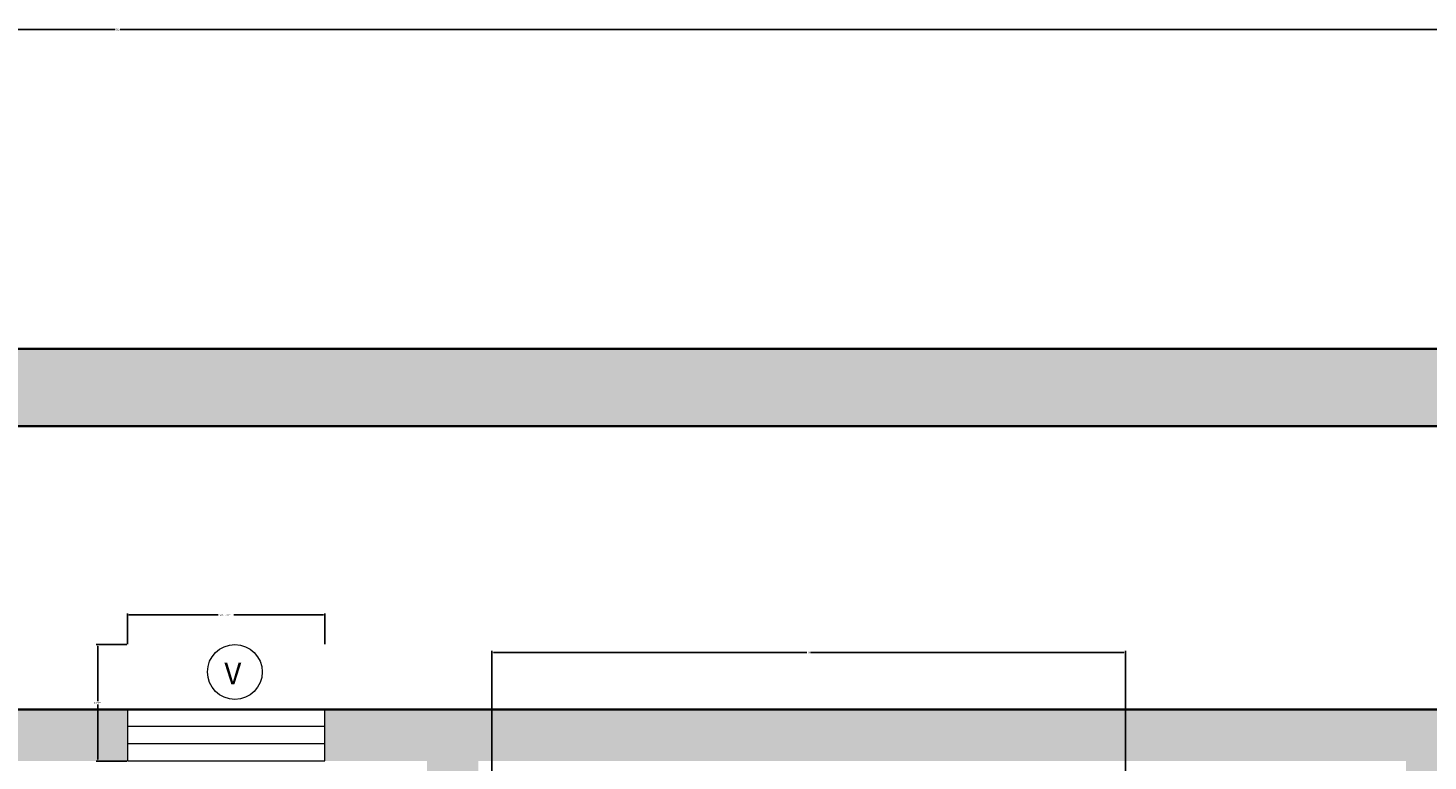
# Model space of a CAD drawing. Units: inches. Extents: x 2701 to 6846, y 811 to 2447.
# Tile 19 of 20: x 2926 to 3089, y 1456 to 1541. Entities that reach past the tile are written whole.
import ezdxf

# ---------------------------------------------------------------- set-up
doc = ezdxf.new("R2010")
doc.units = ezdxf.units.IN
for name, color, linetype, lineweight in [('A-ANNO-DIMS', 2, 'Continuous', 18), ('A-GLAZ', 4, 'Continuous', 18), ('A-WALL', 7, 'Continuous', 35), ('C-PROP', 7, 'Continuous', 35)]:
    doc.layers.add(name, color=color, linetype=linetype, lineweight=lineweight)
doc.layers.add('A-WALL-PATT', color=18, linetype='Continuous', lineweight=13, true_color=0x000000)
doc.layers.add('C-PROP-PATT', color=18, linetype='Continuous', lineweight=13, true_color=0x000000)
doc.styles.get("Standard").update_dxf_attribs({"font": 'arial.ttf'})
doc.dimstyles.get("Standard").update_dxf_attribs({"dimtxt": 0.18, "dimasz": 0.18, "dimexe": 0.18, "dimexo": 0.0625, "dimgap": 0.09, "dimtad": 0, "dimtih": 1, "dimtoh": 1, "dimdec": 4, "dimzin": 0, "dimdsep": 46, "dimtxsty": 'Standard', "dimcen": 0.09, "dimadec": 0, "dimazin": 0, "dimtfac": 1, "dimtdec": 4, "dimtofl": 0, "dimtmove": 0, "dimatfit": 3, "dimfxl": 1, "dimtolj": 1, "dimtzin": 0, "dimarcsym": 0})

# ---------------------------------------------------------------- blocks, each defined once
blk = doc.blocks.new('V')
for p, q in [((3304.15, 1279.33), (3281.15, 1279.33)), ((3304.15, 1277.33), (3281.15, 1277.33)), ((3304.15, 1275.33), (3281.15, 1275.33)), ((3281.15, 1273.33), (3304.15, 1273.33))]:
    blk.add_line(p, q)
blk.add_circle((3293.67, 1283.69), 3.19)
at = {"insert": (3292.45, 1284.76), "char_height": 2.5, "attachment_point": 1}
blk.add_mtext_dynamic_manual_height_columns('V', width=0.0153, gutter_width=12.5, heights=[0], dxfattribs=at)
blk = doc.blocks.new('V1')
for p, q in [((3281.15, 1279.33), (3281.15, 1273.33)), ((3304.15, 1273.33), (3304.15, 1279.33))]:
    blk.add_line(p, q)
blk.add_blockref('V', (0, 0))
blk = doc.blocks.new('*D37')
at = {"layer": 'A-ANNO-DIMS', "color": 0, "lineweight": -2, "transparency": 16777216}
for p, q in [((2937.09, 1469.67), (2937.09, 1473.24)), ((2937.27, 1473.06), (2947.68, 1473.06)), ((2959.91, 1473.06), (2949.49, 1473.06)), ((2960.09, 1469.67), (2960.09, 1473.24))]:
    blk.add_line(p, q, dxfattribs=at)
at = {"layer": 'A-ANNO-DIMS', "color": 0, "transparency": 16777216}
for points in [[(2937.27, 1473.09), (2937.27, 1473.03), (2937.09, 1473.06)], [(2959.91, 1473.09), (2959.91, 1473.03), (2960.09, 1473.06)]]:
    blk.add_solid(points, dxfattribs=at)
at = {"layer": 'Defpoints', "color": 0, "transparency": 16777216}
for p in [(2960.09, 1473.06), (2937.09, 1469.61), (2960.09, 1469.61)]:
    blk.add_point(p, dxfattribs=at)
at = {"layer": 'A-ANNO-DIMS', "color": 0, "transparency": 16777216, "insert": (2948.59, 1473.06), "char_height": 0.18, "attachment_point": 5}
blk.add_mtext('\\A1;VENT 23 TYP.', dxfattribs=at)
blk = doc.blocks.new('*D38')
at = {"layer": 'A-ANNO-DIMS', "color": 0, "lineweight": -2, "transparency": 16777216}
for p, q in [((2937.02, 1469.61), (2933.46, 1469.61)), ((2933.64, 1469.43), (2933.64, 1463.01)), ((2933.64, 1456.23), (2933.64, 1462.65)), ((2937.02, 1456.05), (2933.46, 1456.05))]:
    blk.add_line(p, q, dxfattribs=at)
at = {"layer": 'A-ANNO-DIMS', "color": 0, "transparency": 16777216}
for points in [[(2933.61, 1469.43), (2933.67, 1469.43), (2933.64, 1469.61)], [(2933.61, 1456.23), (2933.67, 1456.23), (2933.64, 1456.05)]]:
    blk.add_solid(points, dxfattribs=at)
at = {"layer": 'Defpoints', "color": 0, "transparency": 16777216}
for p in [(2933.64, 1469.61), (2937.09, 1469.61), (2937.09, 1456.05)]:
    blk.add_point(p, dxfattribs=at)
at = {"layer": 'A-ANNO-DIMS', "color": 0, "transparency": 16777216, "insert": (2933.64, 1462.83), "char_height": 0.18, "attachment_point": 5}
blk.add_mtext('\\A1;14 TYP.', dxfattribs=at)
blk = doc.blocks.new('*D52')
at = {"layer": 'A-ANNO-DIMS', "color": 0, "lineweight": -2, "transparency": 16777216}
for p, q in [((2979.55, 1454.45), (2979.55, 1468.88)), ((2979.73, 1468.7), (3016.22, 1468.7)), ((3053.14, 1468.7), (3016.65, 1468.7)), ((3053.32, 1454.45), (3053.32, 1468.88))]:
    blk.add_line(p, q, dxfattribs=at)
at = {"layer": 'A-ANNO-DIMS', "color": 0, "transparency": 16777216}
for points in [[(2979.73, 1468.73), (2979.73, 1468.67), (2979.55, 1468.7)], [(3053.14, 1468.73), (3053.14, 1468.67), (3053.32, 1468.7)]]:
    blk.add_solid(points, dxfattribs=at)
at = {"layer": 'Defpoints', "color": 0, "transparency": 16777216}
for p in [(2979.55, 1468.7), (2979.55, 1454.39), (3053.32, 1454.39)]:
    blk.add_point(p, dxfattribs=at)
at = {"layer": 'A-ANNO-DIMS', "color": 0, "transparency": 16777216, "insert": (3016.44, 1468.7), "char_height": 0.18, "attachment_point": 5}
blk.add_mtext('\\A1;74', dxfattribs=at)
blk = doc.blocks.new('*D67')
at = {"layer": 'A-ANNO-DIMS', "color": 0, "lineweight": -2, "transparency": 16777216}
for p, q in [((2779.97, 1462.11), (2779.97, 1541.43)), ((2780.15, 1541.25), (2935.68, 1541.25)), ((3091.79, 1541.25), (2936.26, 1541.25)), ((3091.97, 1462.11), (3091.97, 1541.43))]:
    blk.add_line(p, q, dxfattribs=at)
at = {"layer": 'A-ANNO-DIMS', "color": 0, "transparency": 16777216}
for points in [[(2780.15, 1541.28), (2780.15, 1541.22), (2779.97, 1541.25)], [(3091.79, 1541.28), (3091.79, 1541.22), (3091.97, 1541.25)]]:
    blk.add_solid(points, dxfattribs=at)
at = {"layer": 'Defpoints', "color": 0, "transparency": 16777216}
for p in [(3091.97, 1541.25), (2779.97, 1462.05), (3091.97, 1462.05)]:
    blk.add_point(p, dxfattribs=at)
at = {"layer": 'A-ANNO-DIMS', "color": 0, "transparency": 16777216, "insert": (2935.97, 1541.25), "char_height": 0.18, "attachment_point": 5}
blk.add_mtext('\\A1;312', dxfattribs=at)

msp = doc.modelspace()

# ---------------------------------------------------------------- hatches: boundary and pattern name
at = {"layer": 'A-WALL-PATT'}
h = msp.add_hatch(color=256, dxfattribs=at)
h.dxf.hatch_style = 1
h.paths.add_polyline_path([(3085.97, 1456.05), (3085.97, 1348.05), (3091.97, 1348.05), (3091.97, 1360.05), (3091.97, 1462.05), (2960.09, 1462.05), (2960.09, 1456.05), (2971.97, 1456.05), (2971.97, 1372.05), (2923.97, 1372.05), (2923.97, 1378.05), (2917.97, 1378.05), (2917.97, 1351.05), (2923.97, 1351.05), (2923.97, 1366.05), (2971.97, 1366.05), (2971.97, 1351.05), (2976.77, 1351.05), (2977.97, 1351.05), (2977.97, 1456.05)])
h.paths.add_polyline_path([(2779.97, 1462.05), (2779.97, 1342.05), (2785.97, 1342.05), (2785.97, 1456.05), (2917.97, 1456.05), (2917.97, 1408.05), (2922.33, 1408.05), (2923.97, 1408.05), (2923.97, 1456.05), (2937.09, 1456.05), (2937.09, 1462.05)])
h.paths.add_polyline_path([(2779.97, 1306.05), (2779.97, 1294.24), (2785.97, 1294.24), (2785.97, 1306.05), (2851.37, 1306.05, -0.025815), (2852.62, 1306.11, -0.025815), (2853.87, 1306.05), (2863.97, 1306.05), (2863.97, 1258.05), (2857.97, 1258.05), (2857.97, 1252.05), (2878.97, 1252.05), (2878.97, 1258.05), (2869.97, 1258.05), (2869.97, 1306.05), (2923.97, 1306.05), (2923.97, 1318.05), (2919.17, 1318.05), (2917.97, 1318.05), (2917.97, 1312.05), (2785.97, 1312.05), (2785.97, 1318.05), (2779.97, 1318.05)])
h.paths.add_polyline_path([(2785.97, 1252.05), (2827.97, 1252.05), (2827.97, 1256.41), (2827.97, 1258.05), (2785.97, 1258.05), (2785.97, 1271.24), (2779.97, 1271.24), (2779.97, 1174.05), (2785.97, 1174.05)])
h.paths.add_polyline_path([(2779.97, 1030.05), (2869.97, 1030.05), (2869.97, 1036.05), (2785.97, 1036.05), (2785.97, 1126.05), (2917.97, 1126.05), (2917.97, 1120.05), (2923.97, 1120.05), (2923.97, 1258.05), (2911.97, 1258.05), (2911.97, 1253.25), (2911.97, 1252.05), (2917.97, 1252.05), (2917.97, 1132.05), (2785.97, 1132.05), (2785.97, 1144.05), (2779.97, 1144.05)])
h.paths.add_polyline_path([(2935.97, 1030.05), (2935.97, 1033.05), (2935.97, 1036.05), (2923.97, 1036.05), (2923.97, 1087.05), (2919.17, 1087.05), (2917.97, 1087.05), (2917.97, 1036.05), (2893.97, 1036.05), (2893.97, 1030.05)])
h.paths.add_polyline_path([(2971.97, 1036.05), (2971.97, 1030.05), (3091.97, 1030.05), (3091.97, 1060.05), (3085.97, 1060.05), (3085.97, 1036.05)])
h.paths.add_polyline_path([(3085.97, 1084.05), (3091.97, 1084.05), (3091.97, 1096.05), (3091.97, 1268.89), (3085.97, 1268.89), (3085.97, 1258.05), (3001.97, 1258.05), (3001.97, 1270.05), (2995.97, 1270.05), (2995.97, 1252.05), (3085.97, 1252.05)])
h.paths.add_polyline_path([(3085.97, 1306.05), (3085.97, 1291.89), (3091.97, 1291.89), (3091.97, 1318.05), (3085.97, 1318.05), (3085.97, 1312.05), (2977.97, 1312.05), (2977.97, 1318.05), (2971.97, 1318.05), (2971.97, 1306.05), (2995.97, 1306.05), (2995.97, 1300.05), (3000.33, 1300.05), (3001.97, 1300.05), (3001.97, 1306.05)])
at = {"layer": 'C-PROP-PATT'}
h = msp.add_hatch(color=256, dxfattribs=at)
h.dxf.hatch_style = 1
h.paths.add_polyline_path([(3145.97, 1504.05), (2737.97, 1504.05), (2737.97, 967.05), (2746.97, 967.05), (2746.97, 1495.05), (3136.97, 1495.05), (3136.97, 865.05), (3130.97, 865.05), (3130.97, 856.05), (3145.97, 856.05)])
h.paths.add_polyline_path([(3070.97, 865.05), (2746.97, 865.05), (2746.97, 871.05), (2737.97, 871.05), (2737.97, 856.05), (3070.97, 856.05)], flags=17)

# ---------------------------------------------------------------- linework, layer by layer
at = {"layer": 'A-WALL'}
msp.add_line((3091.97, 1462.05), (2779.97, 1462.05), dxfattribs=at)
at = {"layer": 'C-PROP'}
for p, q in [((2737.97, 1504.05), (3145.97, 1504.05)), ((2746.97, 1495.05), (3136.97, 1495.05))]:
    msp.add_line(p, q, dxfattribs=at)

# ---------------------------------------------------------------- block references
at = {"layer": 'A-GLAZ'}
msp.add_blockref('V1', (-344.06, 182.73), dxfattribs=at)

# ---------------------------------------------------------------- dimensions: what is measured, and where the dimension line sits
at = {"layer": 'A-ANNO-DIMS'}
dim = msp.add_linear_dim(base=(3091.97, 1541.25), p1=(2779.97, 1462.05), p2=(3091.97, 1462.05), dimstyle='Standard', override={"dimdec": 0, "dimlfac": 1, "dimrnd": 0, "dimzin": 0, "dimdsep": 46, "dimlunit": 2}, dxfattribs=at)
dim.commit()
dim.dimension.update_dxf_attribs({"geometry": '*D67', "text_midpoint": (2935.97, 1541.25)})
dim = msp.add_linear_dim(base=(2960.09, 1473.06), p1=(2937.09, 1469.61), p2=(2960.09, 1469.61), text='VENT <> TYP.', dimstyle='Standard', override={"dimdec": 0, "dimlfac": 1, "dimrnd": 0, "dimzin": 0, "dimdsep": 46, "dimlunit": 2}, dxfattribs=at)
dim.commit()
dim.dimension.update_dxf_attribs({"geometry": '*D37', "text_midpoint": (2948.59, 1473.06)})
dim = msp.add_linear_dim(base=(2933.64, 1469.61), p1=(2937.09, 1456.05), p2=(2937.09, 1469.61), angle=90, text='<> TYP.', dimstyle='Standard', override={"dimdec": 0, "dimlfac": 1, "dimrnd": 0, "dimzin": 0, "dimdsep": 46, "dimlunit": 2}, dxfattribs=at)
dim.commit()
dim.dimension.update_dxf_attribs({"geometry": '*D38', "text_midpoint": (2933.64, 1462.83)})
dim = msp.add_linear_dim(base=(2979.55, 1468.7), p1=(3053.32, 1454.39), p2=(2979.55, 1454.39), angle=180, dimstyle='Standard', override={"dimdec": 0, "dimlfac": 1, "dimrnd": 0, "dimzin": 0, "dimdsep": 46, "dimlunit": 2}, dxfattribs=at)
dim.commit()
dim.dimension.update_dxf_attribs({"geometry": '*D52', "text_midpoint": (3016.44, 1468.7)})

doc.saveas('drawing.dxf')
